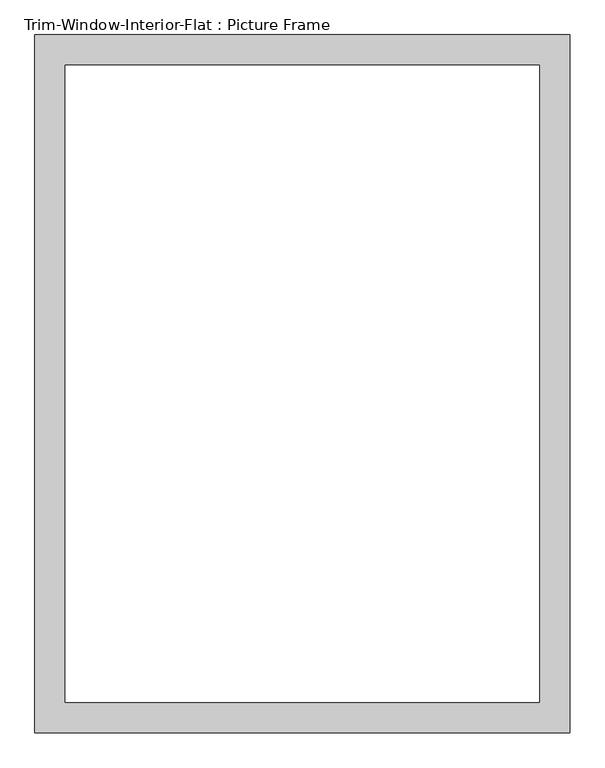
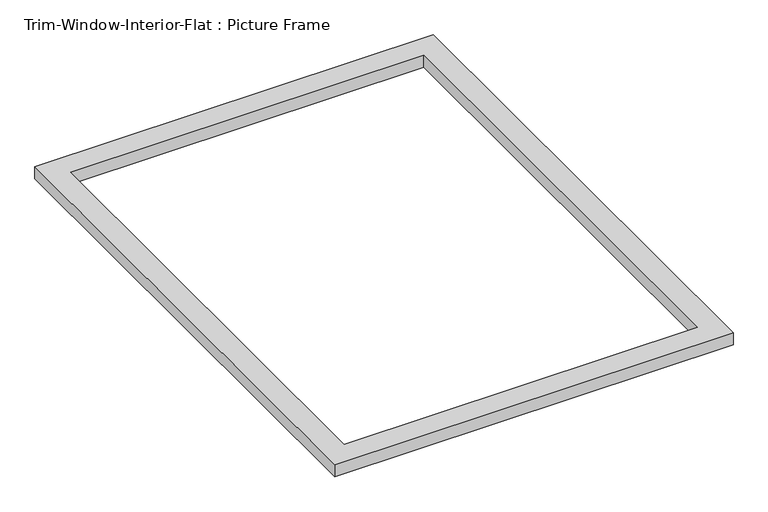
"""IFC4 building model written with IfcOpenShell, lengths in millimetres: proxy geometry, Trim-Window-Interior-Flat : Picture Frame."""

from ifc_helpers import new_model, si_unit, origin, origin_with_axes, place, context, project, spatial, polyline, outline, extrude, source, transform, mapped, element, save


def trim_window_interior_flat_picture_frame_39ff4276(model_context):
    return source(origin(), model_context, "Body", "SweptSolid", [
        extrude(outline(polyline([(501.65, 44.45), (501.65, -1263.65), (-501.65, -1263.65), (-501.65, 44.45), (501.65, 44.45)]), holes=[polyline([(444.5, -12.7), (-444.5, -12.7), (-444.5, -1206.5), (444.5, -1206.5), (444.5, -12.7)])]), origin_with_axes(), (0.0, 0.0, 1.0), 31.75),
    ])


if __name__ == "__main__":
    model = new_model("IFC4")
    model_context = context("Model", 3, world=origin())
    ifc_project = project(units=[si_unit("LENGTHUNIT", "METRE", prefix="MILLI")], contexts=[model_context])
    site = spatial("IfcSite", under=ifc_project)
    building = spatial("IfcBuilding", under=site)
    placement = place(None, origin())
    trim_window_interior_flat_picture_frame_shape = trim_window_interior_flat_picture_frame_39ff4276(model_context)
    element("IfcBuildingElementProxy", 1, Name="Trim-Window-Interior-Flat : Picture Frame", ObjectType="Trim-Window-Interior-Flat : Picture Frame", at=placement, inside=building, context=model_context, shape_type="MappedRepresentation", body=[
        mapped(trim_window_interior_flat_picture_frame_shape, transform((0.0, 0.0, 0.0), x_axis=(1.0, 0.0, 0.0), y_axis=(0.0, 1.0, 0.0), z_axis=(0.0, 0.0, 1.0))),
    ])
    save(model, "model.ifc")

# Revit data of these elements
# Type "Trim-Window-Interior-Flat : Picture Frame"
#   Trim Thickness_Picture Frame = 0' - 1 1/4"
#   Trim Width = 0' - 2 1/4"
#   Trim Thickness_with Sill = 0' - 0 3/4"
#   Sill Thickness = 0' - 1 1/4"
#   Opening Width [instance default] = 2' - 0"
#   Opening Height [instance default] = 3' - 0"
#   Default Elevation = 4' - 0"
#   Sill = no
#   Picture Frame = yes
#   Trim Material [instance default] = none
# Element 1 (IfcBuildingElementProxy, "Trim-Window-Interior-Flat : Picture Frame")
#   Opening Width = 3' - 0"
#   Opening Height = 4' - 0"
#   Trim Material = Wood - Stained
#   Materials on its faces: "Wood - Stained"
# Materials
#   "Wood - Stained": class "Wood", colour RGB 224 178 126, transparency 0, Cost = 0
